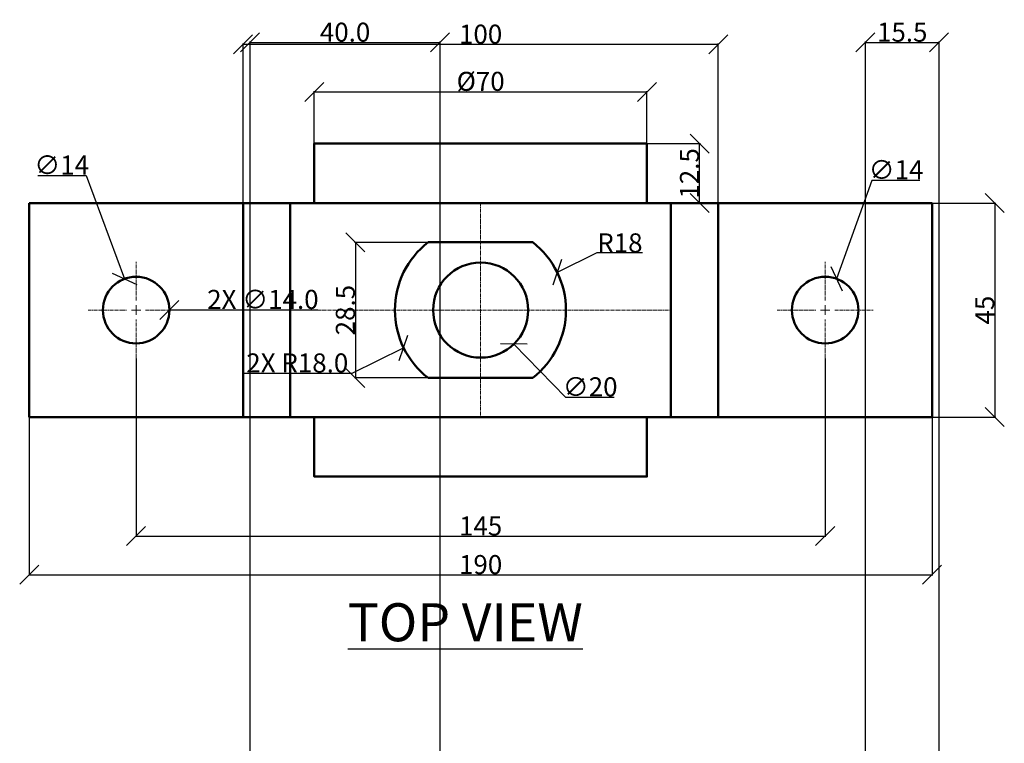
# Model space of a CAD drawing. Units: millimetres. Extents: x 2623 to 3019, y 2308 to 2699.
# Tile 2 of 3: x 2649 to 2856, y 2547 to 2699. Entities that reach past the tile are written whole.
import ezdxf

# ---------------------------------------------------------------- set-up
doc = ezdxf.new("R2010")
doc.units = ezdxf.units.MM
doc.header["$MEASUREMENT"] = 0
doc.linetypes.add('CENTER2', pattern=[1.125, 0.75, -0.125, 0.125, -0.125])
for name, color, linetype, lineweight in [('M-CNTR', 1, 'CENTER2', 18), ('M-DIMS', 2, 'Continuous', 25), ('M-OUTL', 7, 'Continuous', 50), ('M-TEXT', 7, 'Continuous', 25)]:
    doc.layers.add(name, color=color, linetype=linetype, lineweight=lineweight)
doc.styles.get("Standard").update_dxf_attribs({"font": 'arial.ttf'})
doc.dimstyles.get("Standard").update_dxf_attribs({"dimtxt": 4, "dimasz": 4, "dimexe": 0.18, "dimexo": 0.0625, "dimgap": 0.09, "dimtad": 1, "dimtoh": 1, "dimdec": 0, "dimzin": 0, "dimdsep": 46, "dimtxsty": 'Standard', "dimblk": 'OBLIQUE', "dimcen": 0.09, "dimclre": 251, "dimadec": 0, "dimazin": 0, "dimtfac": 1, "dimtdec": 0, "dimtofl": 0, "dimtmove": 0, "dimatfit": 3, "dimfxl": 1, "dimtolj": 1, "dimtzin": 0, "dimarcsym": 0})

# ---------------------------------------------------------------- blocks, each defined once
blk = doc.blocks.new('_Oblique')
at = {"color": 0, "linetype": 'ByBlock', "lineweight": -2}
blk.add_line((-0.5, -0.5), (0.5, 0.5), dxfattribs=at)
blk = doc.blocks.new('*D33')
at = {"layer": 'Defpoints', "color": 0, "transparency": 16777216}
for p in [(2650.62, 2615.84), (2840.62, 2615.84), (2840.62, 2582.7)]:
    blk.add_point(p, dxfattribs=at)
at = {"layer": 'M-DIMS', "color": 0, "lineweight": -2, "transparency": 16777216}
for p, q in [((2650.62, 2615.78), (2650.62, 2582.52)), ((2840.62, 2615.78), (2840.62, 2582.52)), ((2650.62, 2582.7), (2840.62, 2582.7))]:
    blk.add_line(p, q, dxfattribs=at)
at = {"layer": 'M-DIMS', "color": 0, "lineweight": -2, "transparency": 16777216, "xscale": 4, "yscale": 4, "zscale": 4, "rotation": 180}
blk.add_blockref('_Oblique', (2650.62, 2582.7), dxfattribs=at)
at = {"layer": 'M-DIMS', "color": 0, "lineweight": -2, "transparency": 16777216, "xscale": 4, "yscale": 4, "zscale": 4}
blk.add_blockref('_Oblique', (2840.62, 2582.7), dxfattribs=at)
at = {"layer": 'M-DIMS', "color": 0, "transparency": 16777216, "insert": (2745.62, 2584.83), "char_height": 4, "attachment_point": 5}
blk.add_mtext('\\A1;190', dxfattribs=at)
blk = doc.blocks.new('*U34')
at = {"layer": 'M-CNTR', "color": 0, "transparency": 16777216}
for p, q in [((0, 2), (0, 10.12)), ((-10.12, 0), (-2, 0)), ((2, 0), (10.12, 0)), ((0, -10.12), (0, -2))]:
    blk.add_line(p, q, dxfattribs=at)
at = {"layer": 'M-CNTR', "color": 0, "linetype": 'Continuous', "transparency": 16777216}
for p, q in [((-1, 0), (1, 0)), ((0, -1), (0, 1))]:
    blk.add_line(p, q, dxfattribs=at)
blk = doc.blocks.new('*U35')
at = {"layer": 'M-CNTR', "color": 0, "transparency": 16777216}
for p, q in [((0, 2), (0, 10.12)), ((-10.12, 0), (-2, 0)), ((2, 0), (10.12, 0)), ((0, -10.12), (0, -2))]:
    blk.add_line(p, q, dxfattribs=at)
at = {"layer": 'M-CNTR', "color": 0, "linetype": 'Continuous', "transparency": 16777216}
for p, q in [((-1, 0), (1, 0)), ((0, -1), (0, 1))]:
    blk.add_line(p, q, dxfattribs=at)
blk = doc.blocks.new('*D36')
at = {"layer": 'Defpoints', "color": 0, "transparency": 16777216}
for p in [(2734.58, 2652.59), (2719.28, 2624.09), (2734.58, 2624.09)]:
    blk.add_point(p, dxfattribs=at)
at = {"layer": 'M-DIMS', "color": 0, "lineweight": -2, "transparency": 16777216}
for p, q in [((2734.52, 2652.59), (2719.1, 2652.59)), ((2719.28, 2652.59), (2719.28, 2624.09)), ((2734.52, 2624.09), (2719.1, 2624.09))]:
    blk.add_line(p, q, dxfattribs=at)
at = {"layer": 'M-DIMS', "color": 0, "lineweight": -2, "transparency": 16777216, "xscale": 4, "yscale": 4, "zscale": 4}
for p, rotation in [((2719.28, 2652.59), 90), ((2719.28, 2624.09), 270)]:
    blk.add_blockref('_Oblique', p, dxfattribs=dict(at, rotation=rotation))
at = {"layer": 'M-DIMS', "color": 0, "transparency": 16777216, "insert": (2717.15, 2638.34), "char_height": 4, "attachment_point": 5, "rotation": 90}
blk.add_mtext('\\A1;28.5', dxfattribs=at)
blk = doc.blocks.new('*D37')
at = {"layer": 'Defpoints', "color": 0, "transparency": 16777216}
for p in [(2673.12, 2628.22), (2818.12, 2628.22), (2818.12, 2590.82)]:
    blk.add_point(p, dxfattribs=at)
at = {"layer": 'M-DIMS', "color": 0, "lineweight": -2, "transparency": 16777216}
for p, q in [((2673.12, 2628.16), (2673.12, 2590.64)), ((2818.12, 2628.16), (2818.12, 2590.64)), ((2673.12, 2590.82), (2818.12, 2590.82))]:
    blk.add_line(p, q, dxfattribs=at)
at = {"layer": 'M-DIMS', "color": 0, "lineweight": -2, "transparency": 16777216, "xscale": 4, "yscale": 4, "zscale": 4, "rotation": 180}
blk.add_blockref('_Oblique', (2673.12, 2590.82), dxfattribs=at)
at = {"layer": 'M-DIMS', "color": 0, "lineweight": -2, "transparency": 16777216, "xscale": 4, "yscale": 4, "zscale": 4}
blk.add_blockref('_Oblique', (2818.12, 2590.82), dxfattribs=at)
at = {"layer": 'M-DIMS', "color": 0, "transparency": 16777216, "insert": (2745.62, 2592.95), "char_height": 4, "attachment_point": 5}
blk.add_mtext('\\A1;145', dxfattribs=at)
blk = doc.blocks.new('*D38')
at = {"layer": 'Defpoints', "color": 0, "transparency": 16777216}
for p in [(2780.62, 2673.34), (2791.69, 2673.34), (2780.62, 2660.84)]:
    blk.add_point(p, dxfattribs=at)
at = {"layer": 'M-DIMS', "color": 0, "lineweight": -2, "transparency": 16777216}
for p, q in [((2780.69, 2673.34), (2791.87, 2673.34)), ((2791.69, 2660.84), (2791.69, 2673.34)), ((2780.69, 2660.84), (2791.87, 2660.84))]:
    blk.add_line(p, q, dxfattribs=at)
at = {"layer": 'M-DIMS', "color": 0, "lineweight": -2, "transparency": 16777216, "xscale": 4, "yscale": 4, "zscale": 4}
for p, rotation in [((2791.69, 2673.34), 90), ((2791.69, 2660.84), 270)]:
    blk.add_blockref('_Oblique', p, dxfattribs=dict(at, rotation=rotation))
at = {"layer": 'M-DIMS', "color": 0, "transparency": 16777216, "insert": (2789.56, 2667.09), "char_height": 4, "attachment_point": 5, "rotation": 90}
blk.add_mtext('\\A1;12.5', dxfattribs=at)
blk = doc.blocks.new('*D39')
at = {"layer": 'Defpoints', "color": 0, "transparency": 16777216}
for p in [(2840.62, 2660.84), (2840.62, 2615.84), (2853.82, 2615.84)]:
    blk.add_point(p, dxfattribs=at)
at = {"layer": 'M-DIMS', "color": 0, "lineweight": -2, "transparency": 16777216}
for p, q in [((2840.69, 2660.84), (2854, 2660.84)), ((2853.82, 2660.84), (2853.82, 2615.84)), ((2840.69, 2615.84), (2854, 2615.84))]:
    blk.add_line(p, q, dxfattribs=at)
at = {"layer": 'M-DIMS', "color": 0, "lineweight": -2, "transparency": 16777216, "xscale": 4, "yscale": 4, "zscale": 4}
for p, rotation in [((2853.82, 2660.84), 90), ((2853.82, 2615.84), 270)]:
    blk.add_blockref('_Oblique', p, dxfattribs=dict(at, rotation=rotation))
at = {"layer": 'M-DIMS', "color": 0, "transparency": 16777216, "insert": (2851.69, 2638.34), "char_height": 4, "attachment_point": 5, "rotation": 90}
blk.add_mtext('\\A1;45', dxfattribs=at)
blk = doc.blocks.new('*D40')
at = {"layer": 'Defpoints', "color": 0, "transparency": 16777216}
for p in [(2710.62, 2684.19), (2710.62, 2673.34), (2780.62, 2673.34)]:
    blk.add_point(p, dxfattribs=at)
at = {"layer": 'M-DIMS', "color": 0, "lineweight": -2, "transparency": 16777216}
for p, q in [((2710.62, 2673.41), (2710.62, 2684.37)), ((2780.62, 2684.19), (2710.62, 2684.19)), ((2780.62, 2673.41), (2780.62, 2684.37))]:
    blk.add_line(p, q, dxfattribs=at)
at = {"layer": 'M-DIMS', "color": 0, "lineweight": -2, "transparency": 16777216, "xscale": 4, "yscale": 4, "zscale": 4, "rotation": 180}
blk.add_blockref('_Oblique', (2710.62, 2684.19), dxfattribs=at)
at = {"layer": 'M-DIMS', "color": 0, "lineweight": -2, "transparency": 16777216, "xscale": 4, "yscale": 4, "zscale": 4}
blk.add_blockref('_Oblique', (2780.62, 2684.19), dxfattribs=at)
at = {"layer": 'M-DIMS', "color": 0, "transparency": 16777216, "insert": (2745.62, 2686.44), "char_height": 4, "attachment_point": 5}
blk.add_mtext('\\A1;%%C70', dxfattribs=at)
blk = doc.blocks.new('*D41')
at = {"layer": 'Defpoints', "color": 0, "transparency": 16777216}
for p in [(2795.62, 2694.23), (2695.62, 2660.84), (2795.62, 2660.84)]:
    blk.add_point(p, dxfattribs=at)
at = {"layer": 'M-DIMS', "color": 0, "lineweight": -2, "transparency": 16777216}
for p, q in [((2695.62, 2660.91), (2695.62, 2694.41)), ((2695.62, 2694.23), (2795.62, 2694.23)), ((2795.62, 2660.91), (2795.62, 2694.41))]:
    blk.add_line(p, q, dxfattribs=at)
at = {"layer": 'M-DIMS', "color": 0, "lineweight": -2, "transparency": 16777216, "xscale": 4, "yscale": 4, "zscale": 4, "rotation": 180}
blk.add_blockref('_Oblique', (2695.62, 2694.23), dxfattribs=at)
at = {"layer": 'M-DIMS', "color": 0, "lineweight": -2, "transparency": 16777216, "xscale": 4, "yscale": 4, "zscale": 4}
blk.add_blockref('_Oblique', (2795.62, 2694.23), dxfattribs=at)
at = {"layer": 'M-DIMS', "color": 0, "transparency": 16777216, "insert": (2745.62, 2696.36), "char_height": 4, "attachment_point": 5}
blk.add_mtext('\\A1;100', dxfattribs=at)
blk = doc.blocks.new('*D42')
at = {"layer": 'Defpoints', "color": 0, "transparency": 16777216}
for p in [(2738.64, 2645.5), (2752.61, 2631.18)]:
    blk.add_point(p, dxfattribs=at)
at = {"layer": 'M-DIMS', "color": 0, "lineweight": -2, "transparency": 16777216}
for p, q in [((2745.53, 2638.34), (2745.71, 2638.34)), ((2745.62, 2638.25), (2745.62, 2638.43)), ((2763.55, 2619.96), (2752.61, 2631.18)), ((2773.71, 2619.96), (2763.55, 2619.96))]:
    blk.add_line(p, q, dxfattribs=at)
at = {"layer": 'M-DIMS', "color": 0, "lineweight": -2, "transparency": 16777216, "xscale": 4, "yscale": 4, "zscale": 4, "rotation": 134.2809394780327}
blk.add_blockref('_Oblique', (2752.61, 2631.18), dxfattribs=at)
at = {"layer": 'M-DIMS', "color": 0, "transparency": 16777216, "insert": (2768.67, 2622.21), "char_height": 4, "attachment_point": 5}
blk.add_mtext('\\A1;∅20', dxfattribs=at)
blk = doc.blocks.new('*D43')
at = {"layer": 'Defpoints', "color": 0, "transparency": 16777216}
for p in [(2820.49, 2644.93), (2815.76, 2631.76)]:
    blk.add_point(p, dxfattribs=at)
at = {"layer": 'M-DIMS', "color": 0, "lineweight": -2, "transparency": 16777216}
for p, q in [((2827.92, 2665.6), (2820.49, 2644.93)), ((2838.07, 2665.6), (2827.92, 2665.6)), ((2818.03, 2638.34), (2818.21, 2638.34)), ((2818.12, 2638.25), (2818.12, 2638.43))]:
    blk.add_line(p, q, dxfattribs=at)
at = {"layer": 'M-DIMS', "color": 0, "lineweight": -2, "transparency": 16777216, "xscale": 4, "yscale": 4, "zscale": 4, "rotation": 250.2431364427056}
blk.add_blockref('_Oblique', (2820.49, 2644.93), dxfattribs=at)
at = {"layer": 'M-DIMS', "color": 0, "transparency": 16777216, "insert": (2833.04, 2667.85), "char_height": 4, "attachment_point": 5}
blk.add_mtext('\\A1;∅14', dxfattribs=at)
blk = doc.blocks.new('*D44')
at = {"layer": 'Defpoints', "color": 0, "transparency": 16777216}
for p in [(2670.68, 2644.9), (2675.57, 2631.79)]:
    blk.add_point(p, dxfattribs=at)
at = {"layer": 'M-DIMS', "color": 0, "lineweight": -2, "transparency": 16777216}
for p, q in [((2652.42, 2666.61), (2662.58, 2666.61)), ((2662.58, 2666.61), (2670.68, 2644.9)), ((2673.03, 2638.34), (2673.21, 2638.34)), ((2673.12, 2638.25), (2673.12, 2638.43))]:
    blk.add_line(p, q, dxfattribs=at)
at = {"layer": 'M-DIMS', "color": 0, "lineweight": -2, "transparency": 16777216, "xscale": 4, "yscale": 4, "zscale": 4, "rotation": 290.459343474008}
blk.add_blockref('_Oblique', (2670.68, 2644.9), dxfattribs=at)
at = {"layer": 'M-DIMS', "color": 0, "transparency": 16777216, "insert": (2657.46, 2668.85), "char_height": 4, "attachment_point": 5}
blk.add_mtext('\\A1;∅14', dxfattribs=at)
blk = doc.blocks.new('*D45')
at = {"layer": 'Defpoints', "color": 0, "transparency": 16777216}
for p in [(2761.74, 2646.27), (2745.58, 2638.34)]:
    blk.add_point(p, dxfattribs=at)
at = {"layer": 'M-DIMS', "color": 0, "lineweight": -2, "transparency": 16777216}
for p, q in [((2770.06, 2650.35), (2761.74, 2646.27)), ((2779.71, 2650.35), (2770.06, 2650.35)), ((2745.49, 2638.34), (2745.67, 2638.34)), ((2745.58, 2638.25), (2745.58, 2638.43))]:
    blk.add_line(p, q, dxfattribs=at)
at = {"layer": 'M-DIMS', "color": 0, "lineweight": -2, "transparency": 16777216, "xscale": 4, "yscale": 4, "zscale": 4, "rotation": 206.1265183056972}
blk.add_blockref('_Oblique', (2761.74, 2646.27), dxfattribs=at)
at = {"layer": 'M-DIMS', "color": 0, "transparency": 16777216, "insert": (2774.93, 2652.48), "char_height": 4, "attachment_point": 5}
blk.add_mtext('\\A1;R18', dxfattribs=at)
blk = doc.blocks.new('*D49')
at = {"layer": 'Defpoints', "color": 0, "transparency": 16777216}
for p in [(2842.09, 2694.64), (2826.59, 2389.31), (2842.09, 2389.31)]:
    blk.add_point(p, dxfattribs=at)
at = {"layer": 'M-DIMS', "color": 251, "lineweight": -2, "transparency": 16777216}
for p, q in [((2826.59, 2389.37), (2826.59, 2694.82)), ((2842.09, 2389.37), (2842.09, 2694.82))]:
    blk.add_line(p, q, dxfattribs=at)
at = {"layer": 'M-DIMS', "color": 0, "lineweight": -2, "transparency": 16777216}
blk.add_line((2826.59, 2694.64), (2842.09, 2694.64), dxfattribs=at)
at = {"layer": 'M-DIMS', "color": 0, "lineweight": -2, "transparency": 16777216, "xscale": 4, "yscale": 4, "zscale": 4, "rotation": 180}
blk.add_blockref('_Oblique', (2826.59, 2694.64), dxfattribs=at)
at = {"layer": 'M-DIMS', "color": 0, "lineweight": -2, "transparency": 16777216, "xscale": 4, "yscale": 4, "zscale": 4}
blk.add_blockref('_Oblique', (2842.09, 2694.64), dxfattribs=at)
at = {"layer": 'M-DIMS', "color": 0, "transparency": 16777216, "insert": (2834.34, 2696.78), "char_height": 4, "attachment_point": 5}
blk.add_mtext('\\A1;15.5', dxfattribs=at)
blk = doc.blocks.new('*D52')
at = {"layer": 'Defpoints', "color": 0, "transparency": 16777216}
for p in [(2737.09, 2694.64), (2737.09, 2529.31), (2697.09, 2439.31)]:
    blk.add_point(p, dxfattribs=at)
at = {"layer": 'M-DIMS', "color": 251, "lineweight": -2, "transparency": 16777216}
for p, q in [((2697.09, 2439.37), (2697.09, 2694.82)), ((2737.09, 2529.37), (2737.09, 2694.82))]:
    blk.add_line(p, q, dxfattribs=at)
at = {"layer": 'M-DIMS', "color": 0, "lineweight": -2, "transparency": 16777216}
blk.add_line((2697.09, 2694.64), (2737.09, 2694.64), dxfattribs=at)
at = {"layer": 'M-DIMS', "color": 0, "lineweight": -2, "transparency": 16777216, "xscale": 4, "yscale": 4, "zscale": 4, "rotation": 180}
blk.add_blockref('_Oblique', (2697.09, 2694.64), dxfattribs=at)
at = {"layer": 'M-DIMS', "color": 0, "lineweight": -2, "transparency": 16777216, "xscale": 4, "yscale": 4, "zscale": 4}
blk.add_blockref('_Oblique', (2737.09, 2694.64), dxfattribs=at)
at = {"layer": 'M-DIMS', "color": 0, "transparency": 16777216, "insert": (2717.09, 2696.78), "char_height": 4, "attachment_point": 5}
blk.add_mtext('\\A1;40.0', dxfattribs=at)
blk = doc.blocks.new('*D54')
at = {"layer": 'Defpoints', "color": 0, "transparency": 16777216}
for p in [(2745.58, 2638.34), (2729.41, 2630.42)]:
    blk.add_point(p, dxfattribs=at)
at = {"layer": 'M-DIMS', "color": 251, "lineweight": -2, "transparency": 16777216}
for p, q in [((2745.49, 2638.34), (2745.67, 2638.34)), ((2745.58, 2638.25), (2745.58, 2638.43))]:
    blk.add_line(p, q, dxfattribs=at)
at = {"layer": 'M-DIMS', "color": 0, "lineweight": -2, "transparency": 16777216}
for p, q in [((2718.56, 2625.1), (2729.41, 2630.42)), ((2695.6, 2625.1), (2718.56, 2625.1))]:
    blk.add_line(p, q, dxfattribs=at)
at = {"layer": 'M-DIMS', "color": 0, "lineweight": -2, "transparency": 16777216, "xscale": 4, "yscale": 4, "zscale": 4, "rotation": 26.11243383537291}
blk.add_blockref('_Oblique', (2729.41, 2630.42), dxfattribs=at)
at = {"layer": 'M-DIMS', "color": 0, "transparency": 16777216, "insert": (2707.04, 2627.23), "char_height": 4, "attachment_point": 5}
blk.add_mtext('\\A1;2X R18.0', dxfattribs=at)
blk = doc.blocks.new('*D56')
at = {"layer": 'Defpoints', "color": 0, "transparency": 16777216}
for p in [(2666.12, 2638.34), (2680.12, 2638.34)]:
    blk.add_point(p, dxfattribs=at)
at = {"layer": 'M-DIMS', "color": 251, "lineweight": -2, "transparency": 16777216}
for p, q in [((2673.03, 2638.34), (2673.21, 2638.34)), ((2673.12, 2638.25), (2673.12, 2638.43))]:
    blk.add_line(p, q, dxfattribs=at)
at = {"layer": 'M-DIMS', "color": 0, "lineweight": -2, "transparency": 16777216}
for p, q in [((2688.12, 2638.34), (2680.12, 2638.34)), ((2711.39, 2638.34), (2688.12, 2638.34))]:
    blk.add_line(p, q, dxfattribs=at)
at = {"layer": 'M-DIMS', "color": 0, "lineweight": -2, "transparency": 16777216, "xscale": 4, "yscale": 4, "zscale": 4, "rotation": 180.0014569498235}
blk.add_blockref('_Oblique', (2680.12, 2638.34), dxfattribs=at)
at = {"layer": 'M-DIMS', "color": 0, "transparency": 16777216, "insert": (2699.8, 2640.59), "char_height": 4, "attachment_point": 5}
blk.add_mtext('\\A1;2X ∅14.0', dxfattribs=at)

msp = doc.modelspace()

# ---------------------------------------------------------------- linework, layer by layer
at = {"layer": 'M-CNTR'}
for p, q in [((2745.624, 2660.844), (2745.624, 2615.844)), ((2705.526, 2638.344), (2785.624, 2638.344))]:
    msp.add_line(p, q, dxfattribs=at)
at = {"layer": 'M-OUTL'}
for p, q in [((2840.624, 2660.844), (2650.624, 2660.844)), ((2650.624, 2660.844), (2650.624, 2615.844)), ((2695.624, 2660.844), (2695.624, 2615.844)), ((2705.526, 2660.844), (2705.526, 2615.844)), ((2785.624, 2660.844), (2785.624, 2615.844)), ((2795.624, 2660.844), (2795.624, 2615.844)), ((2840.624, 2615.844), (2840.624, 2660.844)), ((2734.578, 2652.594), (2756.572, 2652.594)), ((2734.578, 2624.094), (2756.572, 2624.094)), ((2650.624, 2615.844), (2840.624, 2615.844))]:
    msp.add_line(p, q, dxfattribs=at)
for points in [[(2710.624, 2673.344), (2780.624, 2673.344), (2780.624, 2660.844), (2710.624, 2660.844)], [(2710.624, 2615.844), (2780.624, 2615.844), (2780.624, 2603.344), (2710.624, 2603.344)]]:
    msp.add_lwpolyline(points, close=True, dxfattribs=at)
for centre, radius in [((2745.624, 2638.344), 10), ((2673.124, 2638.344), 7), ((2818.124, 2638.344), 7)]:
    msp.add_circle(centre, radius, dxfattribs=at)
for start, end in [(127.65846, 232.34154), (307.65846, 52.34154)]:
    msp.add_arc((2745.575, 2638.344), 18, start, end, dxfattribs=at)

# ---------------------------------------------------------------- block references
at = {"layer": 'M-CNTR'}
for name, p in [('*U35', (2673.124, 2638.344)), ('*U34', (2818.124, 2638.344))]:
    msp.add_blockref(name, p, dxfattribs=at)

# ---------------------------------------------------------------- texts
at = {"layer": 'M-TEXT', "insert": (2717.653, 2576.705), "char_height": 8, "attachment_point": 1}
msp.add_mtext_dynamic_manual_height_columns('{\\LTOP VIEW}', width=72.37298, gutter_width=1, heights=[0], dxfattribs=at)

# ---------------------------------------------------------------- dimensions: what is measured, and where the dimension line sits
at = {"layer": 'M-DIMS'}
for base, p1, p2, override, picture, middle in [((2795.624, 2694.231), (2695.624, 2660.844), (2795.624, 2660.844), {"dimclrd": 0, "dimclre": 0, "dimclrt": 0}, '*D41', (2745.624, 2696.364)), ((2737.091, 2694.644), (2697.091, 2439.311), (2737.091, 2529.311), {"dimdec": 1, "dimlfac": 1, "dimrnd": 0, "dimzin": 0, "dimdsep": 46, "dimlunit": 2}, '*D52', (2717.091, 2696.776)), ((2842.091, 2694.644), (2826.591, 2389.311), (2842.091, 2389.311), {"dimdec": 1, "dimlfac": 1, "dimrnd": 0, "dimzin": 0, "dimdsep": 46, "dimlunit": 2}, '*D49', (2834.341, 2696.776)), ((2818.124, 2590.822), (2673.124, 2628.224), (2818.124, 2628.224), {"dimclrd": 0, "dimclre": 0, "dimclrt": 0}, '*D37', (2745.624, 2592.954)), ((2840.624, 2582.698), (2650.624, 2615.844), (2840.624, 2615.844), {"dimclrd": 0, "dimclre": 0, "dimclrt": 0}, '*D33', (2745.624, 2584.83))]:
    dim = msp.add_linear_dim(base=base, p1=p1, p2=p2, dimstyle='Standard', override=override, dxfattribs=at)
    dim.commit()
    dim.dimension.update_dxf_attribs({"geometry": picture, "text_midpoint": middle})
dim = msp.add_linear_dim(base=(2710.624, 2684.193), p1=(2780.624, 2673.344), p2=(2710.624, 2673.344), text='%%C<>', dimstyle='Standard', override={"dimclrd": 0, "dimclre": 0, "dimclrt": 0}, dxfattribs=at)
dim.commit()
dim.dimension.update_dxf_attribs({"geometry": '*D40', "text_midpoint": (2745.624, 2686.437)})
for base, p1, p2, override, picture, middle in [((2791.692, 2673.344), (2780.624, 2660.844), (2780.624, 2673.344), {"dimdec": 1, "dimclrd": 0, "dimclre": 0, "dimclrt": 0}, '*D38', (2789.56, 2667.094)), ((2853.817, 2615.844), (2840.624, 2660.844), (2840.624, 2615.844), {"dimclrd": 0, "dimclre": 0, "dimclrt": 0}, '*D39', (2851.693, 2638.344)), ((2719.278, 2624.094), (2734.578, 2652.594), (2734.578, 2624.094), {"dimdec": 1, "dimclrd": 0, "dimclre": 0, "dimclrt": 0}, '*D36', (2717.146, 2638.344))]:
    dim = msp.add_linear_dim(base=base, p1=p1, p2=p2, angle=90, dimstyle='Standard', override=override, dxfattribs=at)
    dim.commit()
    dim.dimension.update_dxf_attribs({"geometry": picture, "text_midpoint": middle})
for p1, p2, picture, middle in [((2675.571, 2631.785), (2670.677, 2644.902), '*D44', (2657.456, 2666.61)), ((2815.758, 2631.756), (2820.49, 2644.932), '*D43', (2833.038, 2665.604)), ((2738.642, 2645.503), (2752.606, 2631.185), '*D42', (2768.672, 2619.965))]:
    dim = msp.add_diameter_dim_2p(p1=p1, p2=p2, dimstyle='Standard', override={"dimclrd": 0, "dimclre": 0, "dimclrt": 0}, dxfattribs=at)
    dim.commit()
    dim.dimension.update_dxf_attribs({"geometry": picture, "text_midpoint": middle, "dimtype": 163})
dim = msp.add_radius_dim(center=(2745.575, 2638.344), mpoint=(2761.736, 2646.27), dimstyle='Standard', override={"dimclrd": 0, "dimclre": 0, "dimclrt": 0}, dxfattribs=at)
dim.commit()
dim.dimension.update_dxf_attribs({"geometry": '*D45', "text_midpoint": (2774.929, 2650.351), "dimtype": 164})
dim = msp.add_diameter_dim_2p(p1=(2666.124, 2638.344), p2=(2680.124, 2638.344), text='2X <>', dimstyle='Standard', override={"dimdec": 1, "dimlfac": 1, "dimrnd": 0, "dimzin": 0, "dimdsep": 46, "dimlunit": 2}, dxfattribs=at)
dim.commit()
dim.dimension.update_dxf_attribs({"geometry": '*D56', "text_midpoint": (2688.124, 2638.344), "dimtype": 163})
dim = msp.add_radius_dim(center=(2745.575, 2638.344), mpoint=(2729.412, 2630.421), text='2X <>', dimstyle='Standard', override={"dimdec": 1, "dimlfac": 1, "dimrnd": 0, "dimzin": 0, "dimdsep": 46, "dimlunit": 2}, dxfattribs=at)
dim.commit()
dim.dimension.update_dxf_attribs({"geometry": '*D54', "text_midpoint": (2707.038, 2627.235)})

doc.saveas('drawing.dxf')
